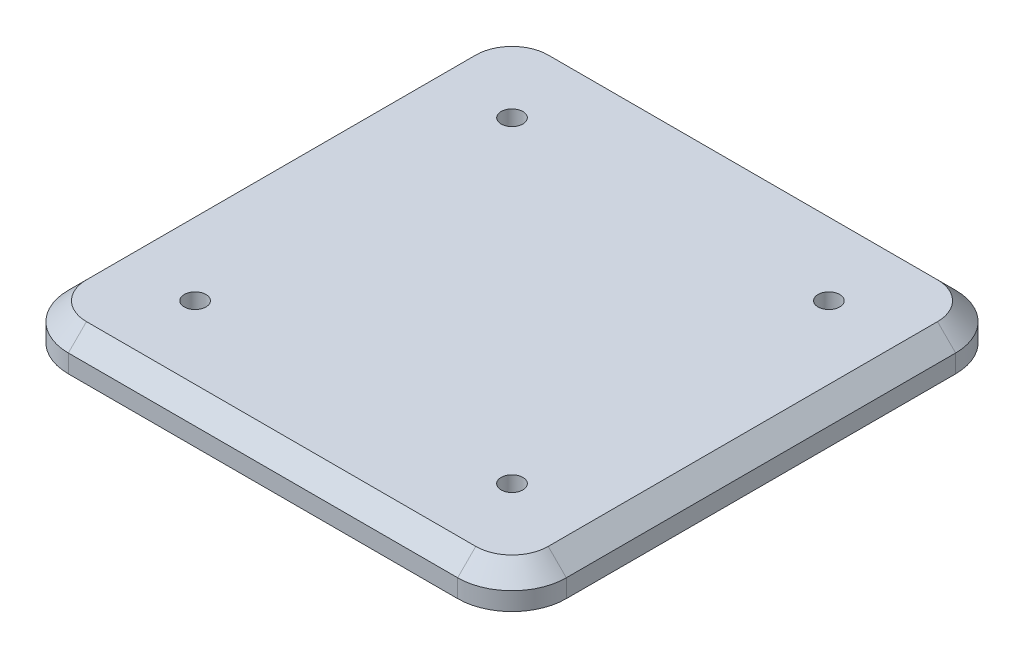
ISO-10303-21;
HEADER;
FILE_DESCRIPTION(('STEP AP214'),'2;1');
FILE_NAME('part.step','',(''),(''),'','','');
FILE_SCHEMA(('AUTOMOTIVE_DESIGN { 1 0 10303 214 1 1 1 1 }'));
ENDSEC;
DATA;
#1=APPLICATION_CONTEXT('core data for automotive mechanical design processes');
#2=APPLICATION_PROTOCOL_DEFINITION('international standard','automotive_design',2000,#1);
#3=PRODUCT_CONTEXT('',#1,'mechanical');
#4=PRODUCT('Part','Part','',(#3));
#5=PRODUCT_RELATED_PRODUCT_CATEGORY('part','',(#4));
#6=PRODUCT_DEFINITION_FORMATION('','',#4);
#7=PRODUCT_DEFINITION_CONTEXT('part definition',#1,'design');
#8=PRODUCT_DEFINITION('design','',#6,#7);
#9=PRODUCT_DEFINITION_SHAPE('','',#8);
#10=(LENGTH_UNIT() NAMED_UNIT(*) SI_UNIT(.MILLI.,.METRE.));
#11=(NAMED_UNIT(*) PLANE_ANGLE_UNIT() SI_UNIT($,.RADIAN.));
#12=(NAMED_UNIT(*) SI_UNIT($,.STERADIAN.) SOLID_ANGLE_UNIT());
#13=UNCERTAINTY_MEASURE_WITH_UNIT(LENGTH_MEASURE(1.E-05),#10,'distance_accuracy_value','');
#14=(GEOMETRIC_REPRESENTATION_CONTEXT(3) GLOBAL_UNCERTAINTY_ASSIGNED_CONTEXT((#13)) GLOBAL_UNIT_ASSIGNED_CONTEXT((#10,
#11,#12)) REPRESENTATION_CONTEXT('',''));
#15=CARTESIAN_POINT('',(0.,0.,0.));
#16=DIRECTION('',(0.,0.,1.));
#17=DIRECTION('',(1.,0.,0.));
#18=AXIS2_PLACEMENT_3D('',#15,#16,#17);
#19=CARTESIAN_POINT('',(-137.5,20.,137.5));
#20=DIRECTION('',(0.,0.,-1.));
#21=DIRECTION('',(-1.,0.,0.));
#22=AXIS2_PLACEMENT_3D('',#19,#20,#21);
#23=PLANE('',#22);
#24=DIRECTION('',(0.,-1.,0.));
#25=VECTOR('',#24,1.);
#26=CARTESIAN_POINT('',(107.5,20.,137.5));
#27=LINE('',#26,#25);
#28=CARTESIAN_POINT('',(107.5,0.,137.5));
#29=VERTEX_POINT('',#28);
#30=CARTESIAN_POINT('',(107.5,9.99999999999999,137.5));
#31=VERTEX_POINT('',#30);
#32=EDGE_CURVE('E249',#29,#31,#27,.F.);
#33=ORIENTED_EDGE('',*,*,#32,.T.);
#34=DIRECTION('',(-1.,0.,0.));
#35=VECTOR('',#34,1.);
#36=CARTESIAN_POINT('',(-107.5,9.99999999999999,137.5));
#37=LINE('',#36,#35);
#38=CARTESIAN_POINT('',(-107.5,9.99999999999999,137.5));
#39=VERTEX_POINT('',#38);
#40=EDGE_CURVE('E11',#31,#39,#37,.T.);
#41=ORIENTED_EDGE('',*,*,#40,.T.);
#42=DIRECTION('',(0.,-1.,0.));
#43=VECTOR('',#42,1.);
#44=CARTESIAN_POINT('',(-107.5,0.,137.5));
#45=LINE('',#44,#43);
#46=CARTESIAN_POINT('',(-107.5,0.,137.5));
#47=VERTEX_POINT('',#46);
#48=EDGE_CURVE('E250',#39,#47,#45,.T.);
#49=ORIENTED_EDGE('',*,*,#48,.T.);
#50=DIRECTION('',(1.,0.,0.));
#51=VECTOR('',#50,1.);
#52=CARTESIAN_POINT('',(-137.5,0.,137.5));
#53=LINE('',#52,#51);
#54=EDGE_CURVE('E215',#47,#29,#53,.T.);
#55=ORIENTED_EDGE('',*,*,#54,.T.);
#56=EDGE_LOOP('',(#33,#41,#49,#55));
#57=FACE_BOUND('',#56,.T.);
#58=ADVANCED_FACE('F41',(#57),#23,.F.);
#59=CARTESIAN_POINT('',(137.5,20.,137.5));
#60=DIRECTION('',(-1.,0.,0.));
#61=DIRECTION('',(0.,0.,1.));
#62=AXIS2_PLACEMENT_3D('',#59,#60,#61);
#63=PLANE('',#62);
#64=DIRECTION('',(0.,-1.,0.));
#65=VECTOR('',#64,1.);
#66=CARTESIAN_POINT('',(137.5,20.,-107.5));
#67=LINE('',#66,#65);
#68=CARTESIAN_POINT('',(137.5,0.,-107.5));
#69=VERTEX_POINT('',#68);
#70=CARTESIAN_POINT('',(137.5,9.99999999999999,-107.5));
#71=VERTEX_POINT('',#70);
#72=EDGE_CURVE('E239',#69,#71,#67,.F.);
#73=ORIENTED_EDGE('',*,*,#72,.T.);
#74=DIRECTION('',(0.,0.,1.));
#75=VECTOR('',#74,1.);
#76=CARTESIAN_POINT('',(137.5,9.99999999999999,107.5));
#77=LINE('',#76,#75);
#78=CARTESIAN_POINT('',(137.5,9.99999999999999,107.5));
#79=VERTEX_POINT('',#78);
#80=EDGE_CURVE('E280',#71,#79,#77,.T.);
#81=ORIENTED_EDGE('',*,*,#80,.T.);
#82=DIRECTION('',(0.,-1.,0.));
#83=VECTOR('',#82,1.);
#84=CARTESIAN_POINT('',(137.5,20.,107.5));
#85=LINE('',#84,#83);
#86=CARTESIAN_POINT('',(137.5,0.,107.5));
#87=VERTEX_POINT('',#86);
#88=EDGE_CURVE('E240',#79,#87,#85,.T.);
#89=ORIENTED_EDGE('',*,*,#88,.T.);
#90=DIRECTION('',(0.,0.,-1.));
#91=VECTOR('',#90,1.);
#92=CARTESIAN_POINT('',(137.5,0.,137.5));
#93=LINE('',#92,#91);
#94=EDGE_CURVE('E214',#87,#69,#93,.T.);
#95=ORIENTED_EDGE('',*,*,#94,.T.);
#96=EDGE_LOOP('',(#73,#81,#89,#95));
#97=FACE_BOUND('',#96,.T.);
#98=ADVANCED_FACE('F349',(#97),#63,.F.);
#99=CARTESIAN_POINT('',(-137.5,20.,-137.5));
#100=DIRECTION('',(0.,0.,-1.));
#101=DIRECTION('',(-1.,0.,0.));
#102=AXIS2_PLACEMENT_3D('',#99,#100,#101);
#103=PLANE('',#102);
#104=DIRECTION('',(0.,-1.,0.));
#105=VECTOR('',#104,1.);
#106=CARTESIAN_POINT('',(-107.5,20.,-137.5));
#107=LINE('',#106,#105);
#108=CARTESIAN_POINT('',(-107.5,0.,-137.5));
#109=VERTEX_POINT('',#108);
#110=CARTESIAN_POINT('',(-107.5,9.99999999999999,-137.5));
#111=VERTEX_POINT('',#110);
#112=EDGE_CURVE('E221',#109,#111,#107,.F.);
#113=ORIENTED_EDGE('',*,*,#112,.T.);
#114=DIRECTION('',(1.,0.,0.));
#115=VECTOR('',#114,1.);
#116=CARTESIAN_POINT('',(-137.5,9.99999999999999,-137.5));
#117=LINE('',#116,#115);
#118=CARTESIAN_POINT('',(107.5,9.99999999999999,-137.5));
#119=VERTEX_POINT('',#118);
#120=EDGE_CURVE('E253',#111,#119,#117,.T.);
#121=ORIENTED_EDGE('',*,*,#120,.T.);
#122=DIRECTION('',(0.,-1.,0.));
#123=VECTOR('',#122,1.);
#124=CARTESIAN_POINT('',(107.5,0.,-137.5));
#125=LINE('',#124,#123);
#126=CARTESIAN_POINT('',(107.5,0.,-137.5));
#127=VERTEX_POINT('',#126);
#128=EDGE_CURVE('E230',#119,#127,#125,.T.);
#129=ORIENTED_EDGE('',*,*,#128,.T.);
#130=DIRECTION('',(1.,0.,0.));
#131=VECTOR('',#130,1.);
#132=CARTESIAN_POINT('',(-137.5,0.,-137.5));
#133=LINE('',#132,#131);
#134=EDGE_CURVE('E217',#109,#127,#133,.T.);
#135=ORIENTED_EDGE('',*,*,#134,.F.);
#136=EDGE_LOOP('',(#113,#121,#129,#135));
#137=FACE_BOUND('',#136,.T.);
#138=ADVANCED_FACE('F332',(#137),#103,.T.);
#139=CARTESIAN_POINT('',(-137.5,20.,137.5));
#140=DIRECTION('',(-1.,0.,0.));
#141=DIRECTION('',(0.,0.,1.));
#142=AXIS2_PLACEMENT_3D('',#139,#140,#141);
#143=PLANE('',#142);
#144=DIRECTION('',(0.,-1.,0.));
#145=VECTOR('',#144,1.);
#146=CARTESIAN_POINT('',(-137.5,20.,107.5));
#147=LINE('',#146,#145);
#148=CARTESIAN_POINT('',(-137.5,0.,107.5));
#149=VERTEX_POINT('',#148);
#150=CARTESIAN_POINT('',(-137.5,9.99999999999999,107.5));
#151=VERTEX_POINT('',#150);
#152=EDGE_CURVE('E245',#149,#151,#147,.F.);
#153=ORIENTED_EDGE('',*,*,#152,.T.);
#154=DIRECTION('',(0.,0.,-1.));
#155=VECTOR('',#154,1.);
#156=CARTESIAN_POINT('',(-137.5,9.99999999999999,137.5));
#157=LINE('',#156,#155);
#158=CARTESIAN_POINT('',(-137.5,9.99999999999999,-107.5));
#159=VERTEX_POINT('',#158);
#160=EDGE_CURVE('E274',#151,#159,#157,.T.);
#161=ORIENTED_EDGE('',*,*,#160,.T.);
#162=DIRECTION('',(0.,-1.,0.));
#163=VECTOR('',#162,1.);
#164=CARTESIAN_POINT('',(-137.5,20.,-107.5));
#165=LINE('',#164,#163);
#166=CARTESIAN_POINT('',(-137.5,0.,-107.5));
#167=VERTEX_POINT('',#166);
#168=EDGE_CURVE('E244',#159,#167,#165,.T.);
#169=ORIENTED_EDGE('',*,*,#168,.T.);
#170=DIRECTION('',(0.,0.,-1.));
#171=VECTOR('',#170,1.);
#172=CARTESIAN_POINT('',(-137.5,0.,137.5));
#173=LINE('',#172,#171);
#174=EDGE_CURVE('E222',#149,#167,#173,.T.);
#175=ORIENTED_EDGE('',*,*,#174,.F.);
#176=EDGE_LOOP('',(#153,#161,#169,#175));
#177=FACE_BOUND('',#176,.T.);
#178=ADVANCED_FACE('F345',(#177),#143,.T.);
#179=CARTESIAN_POINT('',(0.,20.,0.));
#180=DIRECTION('',(0.,1.,0.));
#181=DIRECTION('',(0.,0.,1.));
#182=AXIS2_PLACEMENT_3D('',#179,#180,#181);
#183=PLANE('',#182);
#184=CARTESIAN_POINT('',(-87.5,20.,-87.5));
#185=DIRECTION('',(0.,1.,0.));
#186=DIRECTION('',(0.,0.,1.));
#187=AXIS2_PLACEMENT_3D('',#184,#185,#186);
#188=CIRCLE('',#187,5.99999999999999);
#189=CARTESIAN_POINT('',(-87.5,20.,-81.5));
#190=VERTEX_POINT('',#189);
#191=EDGE_CURVE('E190',#190,#190,#188,.T.);
#192=ORIENTED_EDGE('',*,*,#191,.F.);
#193=EDGE_LOOP('',(#192));
#194=FACE_BOUND('',#193,.T.);
#195=CARTESIAN_POINT('',(87.5,20.,-87.5));
#196=DIRECTION('',(0.,1.,0.));
#197=DIRECTION('',(0.,0.,1.));
#198=AXIS2_PLACEMENT_3D('',#195,#196,#197);
#199=CIRCLE('',#198,5.99999999999999);
#200=CARTESIAN_POINT('',(87.5,20.,-81.5));
#201=VERTEX_POINT('',#200);
#202=EDGE_CURVE('E191',#201,#201,#199,.T.);
#203=ORIENTED_EDGE('',*,*,#202,.F.);
#204=EDGE_LOOP('',(#203));
#205=FACE_BOUND('',#204,.T.);
#206=CARTESIAN_POINT('',(87.5,20.,87.5));
#207=DIRECTION('',(0.,1.,0.));
#208=DIRECTION('',(0.,0.,1.));
#209=AXIS2_PLACEMENT_3D('',#206,#207,#208);
#210=CIRCLE('',#209,5.99999999999999);
#211=CARTESIAN_POINT('',(87.5,20.,93.5));
#212=VERTEX_POINT('',#211);
#213=EDGE_CURVE('E200',#212,#212,#210,.T.);
#214=ORIENTED_EDGE('',*,*,#213,.F.);
#215=EDGE_LOOP('',(#214));
#216=FACE_BOUND('',#215,.T.);
#217=CARTESIAN_POINT('',(-87.5,20.,87.5));
#218=DIRECTION('',(0.,1.,0.));
#219=DIRECTION('',(0.,0.,1.));
#220=AXIS2_PLACEMENT_3D('',#217,#218,#219);
#221=CIRCLE('',#220,5.99999999999999);
#222=CARTESIAN_POINT('',(-87.5,20.,93.5));
#223=VERTEX_POINT('',#222);
#224=EDGE_CURVE('E202',#223,#223,#221,.T.);
#225=ORIENTED_EDGE('',*,*,#224,.F.);
#226=EDGE_LOOP('',(#225));
#227=FACE_BOUND('',#226,.T.);
#228=CARTESIAN_POINT('',(107.5,20.,-107.5));
#229=DIRECTION('',(0.,1.,0.));
#230=DIRECTION('',(0.,0.,1.));
#231=AXIS2_PLACEMENT_3D('',#228,#229,#230);
#232=CIRCLE('',#231,20.);
#233=CARTESIAN_POINT('',(127.5,20.,-107.5));
#234=VERTEX_POINT('',#233);
#235=CARTESIAN_POINT('',(107.5,20.,-127.5));
#236=VERTEX_POINT('',#235);
#237=EDGE_CURVE('E262',#234,#236,#232,.T.);
#238=ORIENTED_EDGE('',*,*,#237,.T.);
#239=DIRECTION('',(-1.,0.,0.));
#240=VECTOR('',#239,1.);
#241=CARTESIAN_POINT('',(0.,20.,-127.5));
#242=LINE('',#241,#240);
#243=CARTESIAN_POINT('',(-107.5,20.,-127.5));
#244=VERTEX_POINT('',#243);
#245=EDGE_CURVE('E268',#236,#244,#242,.T.);
#246=ORIENTED_EDGE('',*,*,#245,.T.);
#247=CARTESIAN_POINT('',(-107.5,20.,-107.5));
#248=DIRECTION('',(0.,1.,0.));
#249=DIRECTION('',(0.,0.,1.));
#250=AXIS2_PLACEMENT_3D('',#247,#248,#249);
#251=CIRCLE('',#250,20.);
#252=CARTESIAN_POINT('',(-127.5,20.,-107.5));
#253=VERTEX_POINT('',#252);
#254=EDGE_CURVE('E266',#244,#253,#251,.T.);
#255=ORIENTED_EDGE('',*,*,#254,.T.);
#256=DIRECTION('',(0.,0.,1.));
#257=VECTOR('',#256,1.);
#258=CARTESIAN_POINT('',(-127.5,20.,0.));
#259=LINE('',#258,#257);
#260=CARTESIAN_POINT('',(-127.5,20.,107.5));
#261=VERTEX_POINT('',#260);
#262=EDGE_CURVE('E265',#253,#261,#259,.T.);
#263=ORIENTED_EDGE('',*,*,#262,.T.);
#264=CARTESIAN_POINT('',(-107.5,20.,107.5));
#265=DIRECTION('',(0.,1.,0.));
#266=DIRECTION('',(0.,0.,1.));
#267=AXIS2_PLACEMENT_3D('',#264,#265,#266);
#268=CIRCLE('',#267,20.);
#269=CARTESIAN_POINT('',(-107.5,20.,127.5));
#270=VERTEX_POINT('',#269);
#271=EDGE_CURVE('E256',#261,#270,#268,.T.);
#272=ORIENTED_EDGE('',*,*,#271,.T.);
#273=DIRECTION('',(1.,0.,0.));
#274=VECTOR('',#273,1.);
#275=CARTESIAN_POINT('',(107.5,20.,127.5));
#276=LINE('',#275,#274);
#277=CARTESIAN_POINT('',(107.5,20.,127.5));
#278=VERTEX_POINT('',#277);
#279=EDGE_CURVE('E255',#270,#278,#276,.T.);
#280=ORIENTED_EDGE('',*,*,#279,.T.);
#281=CARTESIAN_POINT('',(107.5,20.,107.5));
#282=DIRECTION('',(0.,1.,0.));
#283=DIRECTION('',(0.,0.,1.));
#284=AXIS2_PLACEMENT_3D('',#281,#282,#283);
#285=CIRCLE('',#284,20.);
#286=CARTESIAN_POINT('',(127.5,20.,107.5));
#287=VERTEX_POINT('',#286);
#288=EDGE_CURVE('E258',#278,#287,#285,.T.);
#289=ORIENTED_EDGE('',*,*,#288,.T.);
#290=DIRECTION('',(0.,0.,-1.));
#291=VECTOR('',#290,1.);
#292=CARTESIAN_POINT('',(127.5,20.,-107.5));
#293=LINE('',#292,#291);
#294=EDGE_CURVE('E257',#287,#234,#293,.T.);
#295=ORIENTED_EDGE('',*,*,#294,.T.);
#296=EDGE_LOOP('',(#238,#246,#255,#263,#272,#280,#289,#295));
#297=FACE_BOUND('',#296,.T.);
#298=ADVANCED_FACE('F313',(#194,#205,#216,#227,#297),#183,.T.);
#299=CARTESIAN_POINT('',(0.,0.,0.));
#300=DIRECTION('',(0.,1.,0.));
#301=DIRECTION('',(0.,0.,1.));
#302=AXIS2_PLACEMENT_3D('',#299,#300,#301);
#303=PLANE('',#302);
#304=CARTESIAN_POINT('',(-112.5,0.,112.5));
#305=DIRECTION('',(0.,-1.,0.));
#306=DIRECTION('',(0.,0.,-1.));
#307=AXIS2_PLACEMENT_3D('',#304,#305,#306);
#308=CIRCLE('',#307,5.99999999999999);
#309=CARTESIAN_POINT('',(-112.5,0.,106.5));
#310=VERTEX_POINT('',#309);
#311=EDGE_CURVE('E164',#310,#310,#308,.T.);
#312=ORIENTED_EDGE('',*,*,#311,.F.);
#313=EDGE_LOOP('',(#312));
#314=FACE_BOUND('',#313,.T.);
#315=CARTESIAN_POINT('',(112.5,0.,112.5));
#316=DIRECTION('',(0.,-1.,0.));
#317=DIRECTION('',(0.,0.,-1.));
#318=AXIS2_PLACEMENT_3D('',#315,#316,#317);
#319=CIRCLE('',#318,5.99999999999999);
#320=CARTESIAN_POINT('',(112.5,0.,106.5));
#321=VERTEX_POINT('',#320);
#322=EDGE_CURVE('E163',#321,#321,#319,.T.);
#323=ORIENTED_EDGE('',*,*,#322,.F.);
#324=EDGE_LOOP('',(#323));
#325=FACE_BOUND('',#324,.T.);
#326=CARTESIAN_POINT('',(112.5,0.,-112.5));
#327=DIRECTION('',(0.,-1.,0.));
#328=DIRECTION('',(0.,0.,-1.));
#329=AXIS2_PLACEMENT_3D('',#326,#327,#328);
#330=CIRCLE('',#329,5.99999999999999);
#331=CARTESIAN_POINT('',(112.5,0.,-118.5));
#332=VERTEX_POINT('',#331);
#333=EDGE_CURVE('E174',#332,#332,#330,.T.);
#334=ORIENTED_EDGE('',*,*,#333,.F.);
#335=EDGE_LOOP('',(#334));
#336=FACE_BOUND('',#335,.T.);
#337=CARTESIAN_POINT('',(-112.5,0.,-112.5));
#338=DIRECTION('',(0.,-1.,0.));
#339=DIRECTION('',(0.,0.,-1.));
#340=AXIS2_PLACEMENT_3D('',#337,#338,#339);
#341=CIRCLE('',#340,5.99999999999999);
#342=CARTESIAN_POINT('',(-112.5,0.,-118.5));
#343=VERTEX_POINT('',#342);
#344=EDGE_CURVE('E182',#343,#343,#341,.T.);
#345=ORIENTED_EDGE('',*,*,#344,.F.);
#346=EDGE_LOOP('',(#345));
#347=FACE_BOUND('',#346,.T.);
#348=ORIENTED_EDGE('',*,*,#134,.T.);
#349=CARTESIAN_POINT('',(107.5,0.,-107.5));
#350=DIRECTION('',(0.,1.,0.));
#351=DIRECTION('',(0.,0.,1.));
#352=AXIS2_PLACEMENT_3D('',#349,#350,#351);
#353=CIRCLE('',#352,30.);
#354=EDGE_CURVE('E232',#127,#69,#353,.F.);
#355=ORIENTED_EDGE('',*,*,#354,.T.);
#356=ORIENTED_EDGE('',*,*,#94,.F.);
#357=CARTESIAN_POINT('',(107.5,0.,107.5));
#358=DIRECTION('',(0.,1.,0.));
#359=DIRECTION('',(0.,0.,1.));
#360=AXIS2_PLACEMENT_3D('',#357,#358,#359);
#361=CIRCLE('',#360,30.);
#362=EDGE_CURVE('E233',#87,#29,#361,.F.);
#363=ORIENTED_EDGE('',*,*,#362,.T.);
#364=ORIENTED_EDGE('',*,*,#54,.F.);
#365=CARTESIAN_POINT('',(-107.5,0.,107.5));
#366=DIRECTION('',(0.,1.,0.));
#367=DIRECTION('',(0.,0.,1.));
#368=AXIS2_PLACEMENT_3D('',#365,#366,#367);
#369=CIRCLE('',#368,30.);
#370=EDGE_CURVE('E227',#47,#149,#369,.F.);
#371=ORIENTED_EDGE('',*,*,#370,.T.);
#372=ORIENTED_EDGE('',*,*,#174,.T.);
#373=CARTESIAN_POINT('',(-107.5,0.,-107.5));
#374=DIRECTION('',(0.,1.,0.));
#375=DIRECTION('',(0.,0.,1.));
#376=AXIS2_PLACEMENT_3D('',#373,#374,#375);
#377=CIRCLE('',#376,30.);
#378=EDGE_CURVE('E231',#167,#109,#377,.F.);
#379=ORIENTED_EDGE('',*,*,#378,.T.);
#380=EDGE_LOOP('',(#348,#355,#356,#363,#364,#371,#372,#379));
#381=FACE_BOUND('',#380,.T.);
#382=ADVANCED_FACE('F333',(#314,#325,#336,#347,#381),#303,.F.);
#383=CARTESIAN_POINT('',(107.5,20.,-107.5));
#384=DIRECTION('',(0.,1.,0.));
#385=DIRECTION('',(0.,0.,1.));
#386=AXIS2_PLACEMENT_3D('',#383,#384,#385);
#387=CYLINDRICAL_SURFACE('',#386,30.);
#388=ORIENTED_EDGE('',*,*,#128,.F.);
#389=CARTESIAN_POINT('',(107.5,9.99999999999999,-107.5));
#390=DIRECTION('',(0.,1.,0.));
#391=DIRECTION('',(0.,0.,1.));
#392=AXIS2_PLACEMENT_3D('',#389,#390,#391);
#393=CIRCLE('',#392,30.);
#394=EDGE_CURVE('E272',#119,#71,#393,.F.);
#395=ORIENTED_EDGE('',*,*,#394,.T.);
#396=ORIENTED_EDGE('',*,*,#72,.F.);
#397=ORIENTED_EDGE('',*,*,#354,.F.);
#398=EDGE_LOOP('',(#388,#395,#396,#397));
#399=FACE_BOUND('',#398,.T.);
#400=ADVANCED_FACE('F355',(#399),#387,.T.);
#401=CARTESIAN_POINT('',(-107.5,20.,-107.5));
#402=DIRECTION('',(0.,-1.,0.));
#403=DIRECTION('',(0.,0.,-1.));
#404=AXIS2_PLACEMENT_3D('',#401,#402,#403);
#405=CYLINDRICAL_SURFACE('',#404,30.);
#406=ORIENTED_EDGE('',*,*,#168,.F.);
#407=CARTESIAN_POINT('',(-107.5,9.99999999999999,-107.5));
#408=DIRECTION('',(0.,1.,0.));
#409=DIRECTION('',(0.,0.,1.));
#410=AXIS2_PLACEMENT_3D('',#407,#408,#409);
#411=CIRCLE('',#410,30.);
#412=EDGE_CURVE('E271',#159,#111,#411,.F.);
#413=ORIENTED_EDGE('',*,*,#412,.T.);
#414=ORIENTED_EDGE('',*,*,#112,.F.);
#415=ORIENTED_EDGE('',*,*,#378,.F.);
#416=EDGE_LOOP('',(#406,#413,#414,#415));
#417=FACE_BOUND('',#416,.T.);
#418=ADVANCED_FACE('F330',(#417),#405,.T.);
#419=CARTESIAN_POINT('',(107.5,20.,107.5));
#420=DIRECTION('',(0.,-1.,0.));
#421=DIRECTION('',(0.,0.,-1.));
#422=AXIS2_PLACEMENT_3D('',#419,#420,#421);
#423=CYLINDRICAL_SURFACE('',#422,30.);
#424=ORIENTED_EDGE('',*,*,#88,.F.);
#425=CARTESIAN_POINT('',(107.5,9.99999999999999,107.5));
#426=DIRECTION('',(0.,1.,0.));
#427=DIRECTION('',(0.,0.,1.));
#428=AXIS2_PLACEMENT_3D('',#425,#426,#427);
#429=CIRCLE('',#428,30.);
#430=EDGE_CURVE('E51',#79,#31,#429,.F.);
#431=ORIENTED_EDGE('',*,*,#430,.T.);
#432=ORIENTED_EDGE('',*,*,#32,.F.);
#433=ORIENTED_EDGE('',*,*,#362,.F.);
#434=EDGE_LOOP('',(#424,#431,#432,#433));
#435=FACE_BOUND('',#434,.T.);
#436=ADVANCED_FACE('F347',(#435),#423,.T.);
#437=CARTESIAN_POINT('',(-107.5,20.,107.5));
#438=DIRECTION('',(0.,1.,0.));
#439=DIRECTION('',(0.,0.,1.));
#440=AXIS2_PLACEMENT_3D('',#437,#438,#439);
#441=CYLINDRICAL_SURFACE('',#440,30.);
#442=ORIENTED_EDGE('',*,*,#48,.F.);
#443=CARTESIAN_POINT('',(-107.5,9.99999999999999,107.5));
#444=DIRECTION('',(0.,1.,0.));
#445=DIRECTION('',(0.,0.,1.));
#446=AXIS2_PLACEMENT_3D('',#443,#444,#445);
#447=CIRCLE('',#446,30.);
#448=EDGE_CURVE('E276',#39,#151,#447,.F.);
#449=ORIENTED_EDGE('',*,*,#448,.T.);
#450=ORIENTED_EDGE('',*,*,#152,.F.);
#451=ORIENTED_EDGE('',*,*,#370,.F.);
#452=EDGE_LOOP('',(#442,#449,#450,#451));
#453=FACE_BOUND('',#452,.T.);
#454=ADVANCED_FACE('F344',(#453),#441,.T.);
#455=CARTESIAN_POINT('',(0.,20.,127.5));
#456=DIRECTION('',(0.,0.707106781186547,0.707106781186547));
#457=DIRECTION('',(-1.,0.,0.));
#458=AXIS2_PLACEMENT_3D('',#455,#456,#457);
#459=PLANE('',#458);
#460=DIRECTION('',(0.,-0.707106781186547,0.707106781186547));
#461=VECTOR('',#460,1.);
#462=CARTESIAN_POINT('',(107.5,20.,127.5));
#463=LINE('',#462,#461);
#464=EDGE_CURVE('E298',#278,#31,#463,.T.);
#465=ORIENTED_EDGE('',*,*,#464,.F.);
#466=ORIENTED_EDGE('',*,*,#279,.F.);
#467=DIRECTION('',(0.,0.707106781186547,-0.707106781186547));
#468=VECTOR('',#467,1.);
#469=CARTESIAN_POINT('',(-107.5,9.99999999999999,137.5));
#470=LINE('',#469,#468);
#471=EDGE_CURVE('E46',#39,#270,#470,.T.);
#472=ORIENTED_EDGE('',*,*,#471,.F.);
#473=ORIENTED_EDGE('',*,*,#40,.F.);
#474=EDGE_LOOP('',(#465,#466,#472,#473));
#475=FACE_BOUND('',#474,.T.);
#476=ADVANCED_FACE('F42',(#475),#459,.T.);
#477=CARTESIAN_POINT('',(-107.5,20.,107.5));
#478=DIRECTION('',(0.,-1.,0.));
#479=DIRECTION('',(0.,0.,-1.));
#480=AXIS2_PLACEMENT_3D('',#477,#478,#479);
#481=CONICAL_SURFACE('',#480,20.,0.785398163397448);
#482=ORIENTED_EDGE('',*,*,#471,.T.);
#483=ORIENTED_EDGE('',*,*,#271,.F.);
#484=DIRECTION('',(0.707106781186547,0.707106781186547,0.));
#485=VECTOR('',#484,1.);
#486=CARTESIAN_POINT('',(-137.5,9.99999999999999,107.5));
#487=LINE('',#486,#485);
#488=EDGE_CURVE('E294',#151,#261,#487,.T.);
#489=ORIENTED_EDGE('',*,*,#488,.F.);
#490=ORIENTED_EDGE('',*,*,#448,.F.);
#491=EDGE_LOOP('',(#482,#483,#489,#490));
#492=FACE_BOUND('',#491,.T.);
#493=ADVANCED_FACE('F308',(#492),#481,.T.);
#494=CARTESIAN_POINT('',(107.5,20.,107.5));
#495=DIRECTION('',(0.,-1.,0.));
#496=DIRECTION('',(0.,0.,-1.));
#497=AXIS2_PLACEMENT_3D('',#494,#495,#496);
#498=CONICAL_SURFACE('',#497,20.,0.785398163397448);
#499=ORIENTED_EDGE('',*,*,#464,.T.);
#500=ORIENTED_EDGE('',*,*,#430,.F.);
#501=DIRECTION('',(0.707106781186547,-0.707106781186547,0.));
#502=VECTOR('',#501,1.);
#503=CARTESIAN_POINT('',(127.5,20.,107.5));
#504=LINE('',#503,#502);
#505=EDGE_CURVE('E292',#287,#79,#504,.T.);
#506=ORIENTED_EDGE('',*,*,#505,.F.);
#507=ORIENTED_EDGE('',*,*,#288,.F.);
#508=EDGE_LOOP('',(#499,#500,#506,#507));
#509=FACE_BOUND('',#508,.T.);
#510=ADVANCED_FACE('F362',(#509),#498,.T.);
#511=CARTESIAN_POINT('',(-137.5,9.99999999999999,137.5));
#512=DIRECTION('',(0.707106781186547,-0.707106781186547,0.));
#513=DIRECTION('',(0.,0.,-1.));
#514=AXIS2_PLACEMENT_3D('',#511,#512,#513);
#515=PLANE('',#514);
#516=ORIENTED_EDGE('',*,*,#488,.T.);
#517=ORIENTED_EDGE('',*,*,#262,.F.);
#518=DIRECTION('',(0.707106781186547,0.707106781186547,0.));
#519=VECTOR('',#518,1.);
#520=CARTESIAN_POINT('',(-137.5,9.99999999999999,-107.5));
#521=LINE('',#520,#519);
#522=EDGE_CURVE('E286',#159,#253,#521,.T.);
#523=ORIENTED_EDGE('',*,*,#522,.F.);
#524=ORIENTED_EDGE('',*,*,#160,.F.);
#525=EDGE_LOOP('',(#516,#517,#523,#524));
#526=FACE_BOUND('',#525,.T.);
#527=ADVANCED_FACE('F320',(#526),#515,.F.);
#528=CARTESIAN_POINT('',(127.5,20.,0.));
#529=DIRECTION('',(0.707106781186547,0.707106781186547,0.));
#530=DIRECTION('',(0.,0.,1.));
#531=AXIS2_PLACEMENT_3D('',#528,#529,#530);
#532=PLANE('',#531);
#533=ORIENTED_EDGE('',*,*,#505,.T.);
#534=ORIENTED_EDGE('',*,*,#80,.F.);
#535=DIRECTION('',(0.707106781186547,-0.707106781186547,0.));
#536=VECTOR('',#535,1.);
#537=CARTESIAN_POINT('',(127.5,20.,-107.5));
#538=LINE('',#537,#536);
#539=EDGE_CURVE('E284',#234,#71,#538,.T.);
#540=ORIENTED_EDGE('',*,*,#539,.F.);
#541=ORIENTED_EDGE('',*,*,#294,.F.);
#542=EDGE_LOOP('',(#533,#534,#540,#541));
#543=FACE_BOUND('',#542,.T.);
#544=ADVANCED_FACE('F363',(#543),#532,.T.);
#545=CARTESIAN_POINT('',(-107.5,20.,-107.5));
#546=DIRECTION('',(0.,-1.,0.));
#547=DIRECTION('',(0.,0.,-1.));
#548=AXIS2_PLACEMENT_3D('',#545,#546,#547);
#549=CONICAL_SURFACE('',#548,20.,0.785398163397448);
#550=ORIENTED_EDGE('',*,*,#522,.T.);
#551=ORIENTED_EDGE('',*,*,#254,.F.);
#552=DIRECTION('',(0.,0.707106781186547,0.707106781186547));
#553=VECTOR('',#552,1.);
#554=CARTESIAN_POINT('',(-107.5,9.99999999999999,-137.5));
#555=LINE('',#554,#553);
#556=EDGE_CURVE('E281',#111,#244,#555,.T.);
#557=ORIENTED_EDGE('',*,*,#556,.F.);
#558=ORIENTED_EDGE('',*,*,#412,.F.);
#559=EDGE_LOOP('',(#550,#551,#557,#558));
#560=FACE_BOUND('',#559,.T.);
#561=ADVANCED_FACE('F321',(#560),#549,.T.);
#562=CARTESIAN_POINT('',(107.5,20.,-107.5));
#563=DIRECTION('',(0.,-1.,0.));
#564=DIRECTION('',(0.,0.,-1.));
#565=AXIS2_PLACEMENT_3D('',#562,#563,#564);
#566=CONICAL_SURFACE('',#565,20.,0.785398163397448);
#567=ORIENTED_EDGE('',*,*,#539,.T.);
#568=ORIENTED_EDGE('',*,*,#394,.F.);
#569=DIRECTION('',(0.,-0.707106781186547,-0.707106781186547));
#570=VECTOR('',#569,1.);
#571=CARTESIAN_POINT('',(107.5,20.,-127.5));
#572=LINE('',#571,#570);
#573=EDGE_CURVE('E211',#236,#119,#572,.T.);
#574=ORIENTED_EDGE('',*,*,#573,.F.);
#575=ORIENTED_EDGE('',*,*,#237,.F.);
#576=EDGE_LOOP('',(#567,#568,#574,#575));
#577=FACE_BOUND('',#576,.T.);
#578=ADVANCED_FACE('F358',(#577),#566,.T.);
#579=CARTESIAN_POINT('',(-137.5,9.99999999999999,-137.5));
#580=DIRECTION('',(0.,-0.707106781186547,0.707106781186547));
#581=DIRECTION('',(1.,0.,0.));
#582=AXIS2_PLACEMENT_3D('',#579,#580,#581);
#583=PLANE('',#582);
#584=ORIENTED_EDGE('',*,*,#556,.T.);
#585=ORIENTED_EDGE('',*,*,#245,.F.);
#586=ORIENTED_EDGE('',*,*,#573,.T.);
#587=ORIENTED_EDGE('',*,*,#120,.F.);
#588=EDGE_LOOP('',(#584,#585,#586,#587));
#589=FACE_BOUND('',#588,.T.);
#590=ADVANCED_FACE('F389',(#589),#583,.F.);
#591=CARTESIAN_POINT('',(-87.5,10.,87.5));
#592=DIRECTION('',(0.,1.,0.));
#593=DIRECTION('',(0.,0.,1.));
#594=AXIS2_PLACEMENT_3D('',#591,#592,#593);
#595=CONICAL_SURFACE('',#594,5.99999999999999,1.02974425867665);
#596=CARTESIAN_POINT('',(-87.5,6.39483628583465,87.5));
#597=VERTEX_POINT('',#596);
#598=VERTEX_LOOP('',#597);
#599=FACE_BOUND('',#598,.T.);
#600=CARTESIAN_POINT('',(-87.5,10.,87.5));
#601=DIRECTION('',(0.,1.,0.));
#602=DIRECTION('',(0.,0.,1.));
#603=AXIS2_PLACEMENT_3D('',#600,#601,#602);
#604=CIRCLE('',#603,5.99999999999999);
#605=CARTESIAN_POINT('',(-87.5,10.,93.5));
#606=VERTEX_POINT('',#605);
#607=EDGE_CURVE('E208',#606,#606,#604,.T.);
#608=ORIENTED_EDGE('',*,*,#607,.T.);
#609=EDGE_LOOP('',(#608));
#610=FACE_BOUND('',#609,.T.);
#611=ADVANCED_FACE('F392',(#599,#610),#595,.F.);
#612=CARTESIAN_POINT('',(-87.5,20.,87.5));
#613=DIRECTION('',(0.,1.,0.));
#614=DIRECTION('',(0.,0.,1.));
#615=AXIS2_PLACEMENT_3D('',#612,#613,#614);
#616=CYLINDRICAL_SURFACE('',#615,5.99999999999999);
#617=ORIENTED_EDGE('',*,*,#607,.F.);
#618=EDGE_LOOP('',(#617));
#619=FACE_BOUND('',#618,.T.);
#620=ORIENTED_EDGE('',*,*,#224,.T.);
#621=EDGE_LOOP('',(#620));
#622=FACE_BOUND('',#621,.T.);
#623=ADVANCED_FACE('F452',(#619,#622),#616,.F.);
#624=CARTESIAN_POINT('',(87.5,10.,87.5));
#625=DIRECTION('',(0.,1.,0.));
#626=DIRECTION('',(0.,0.,1.));
#627=AXIS2_PLACEMENT_3D('',#624,#625,#626);
#628=CONICAL_SURFACE('',#627,5.99999999999999,1.02974425867665);
#629=CARTESIAN_POINT('',(87.5,6.39483628583465,87.5));
#630=VERTEX_POINT('',#629);
#631=VERTEX_LOOP('',#630);
#632=FACE_BOUND('',#631,.T.);
#633=CARTESIAN_POINT('',(87.5,10.,87.5));
#634=DIRECTION('',(0.,1.,0.));
#635=DIRECTION('',(0.,0.,1.));
#636=AXIS2_PLACEMENT_3D('',#633,#634,#635);
#637=CIRCLE('',#636,5.99999999999999);
#638=CARTESIAN_POINT('',(87.5,10.,93.5));
#639=VERTEX_POINT('',#638);
#640=EDGE_CURVE('E205',#639,#639,#637,.T.);
#641=ORIENTED_EDGE('',*,*,#640,.T.);
#642=EDGE_LOOP('',(#641));
#643=FACE_BOUND('',#642,.T.);
#644=ADVANCED_FACE('F462',(#632,#643),#628,.F.);
#645=CARTESIAN_POINT('',(87.5,20.,87.5));
#646=DIRECTION('',(0.,1.,0.));
#647=DIRECTION('',(0.,0.,1.));
#648=AXIS2_PLACEMENT_3D('',#645,#646,#647);
#649=CYLINDRICAL_SURFACE('',#648,5.99999999999999);
#650=ORIENTED_EDGE('',*,*,#640,.F.);
#651=EDGE_LOOP('',(#650));
#652=FACE_BOUND('',#651,.T.);
#653=ORIENTED_EDGE('',*,*,#213,.T.);
#654=EDGE_LOOP('',(#653));
#655=FACE_BOUND('',#654,.T.);
#656=ADVANCED_FACE('F471',(#652,#655),#649,.F.);
#657=CARTESIAN_POINT('',(87.5,10.,-87.5));
#658=DIRECTION('',(0.,1.,0.));
#659=DIRECTION('',(0.,0.,1.));
#660=AXIS2_PLACEMENT_3D('',#657,#658,#659);
#661=CONICAL_SURFACE('',#660,5.99999999999999,1.02974425867665);
#662=CARTESIAN_POINT('',(87.5,6.39483628583465,-87.5));
#663=VERTEX_POINT('',#662);
#664=VERTEX_LOOP('',#663);
#665=FACE_BOUND('',#664,.T.);
#666=CARTESIAN_POINT('',(87.5,10.,-87.5));
#667=DIRECTION('',(0.,1.,0.));
#668=DIRECTION('',(0.,0.,1.));
#669=AXIS2_PLACEMENT_3D('',#666,#667,#668);
#670=CIRCLE('',#669,5.99999999999999);
#671=CARTESIAN_POINT('',(87.5,10.,-81.5));
#672=VERTEX_POINT('',#671);
#673=EDGE_CURVE('E198',#672,#672,#670,.T.);
#674=ORIENTED_EDGE('',*,*,#673,.T.);
#675=EDGE_LOOP('',(#674));
#676=FACE_BOUND('',#675,.T.);
#677=ADVANCED_FACE('F485',(#665,#676),#661,.F.);
#678=CARTESIAN_POINT('',(87.5,20.,-87.5));
#679=DIRECTION('',(0.,1.,0.));
#680=DIRECTION('',(0.,0.,1.));
#681=AXIS2_PLACEMENT_3D('',#678,#679,#680);
#682=CYLINDRICAL_SURFACE('',#681,5.99999999999999);
#683=ORIENTED_EDGE('',*,*,#673,.F.);
#684=EDGE_LOOP('',(#683));
#685=FACE_BOUND('',#684,.T.);
#686=ORIENTED_EDGE('',*,*,#202,.T.);
#687=EDGE_LOOP('',(#686));
#688=FACE_BOUND('',#687,.T.);
#689=ADVANCED_FACE('F491',(#685,#688),#682,.F.);
#690=CARTESIAN_POINT('',(-87.5,10.,-87.5));
#691=DIRECTION('',(0.,1.,0.));
#692=DIRECTION('',(0.,0.,1.));
#693=AXIS2_PLACEMENT_3D('',#690,#691,#692);
#694=CONICAL_SURFACE('',#693,5.99999999999999,1.02974425867665);
#695=CARTESIAN_POINT('',(-87.5,6.39483628583465,-87.5));
#696=VERTEX_POINT('',#695);
#697=VERTEX_LOOP('',#696);
#698=FACE_BOUND('',#697,.T.);
#699=CARTESIAN_POINT('',(-87.5,10.,-87.5));
#700=DIRECTION('',(0.,1.,0.));
#701=DIRECTION('',(0.,0.,1.));
#702=AXIS2_PLACEMENT_3D('',#699,#700,#701);
#703=CIRCLE('',#702,5.99999999999999);
#704=CARTESIAN_POINT('',(-87.5,10.,-81.5));
#705=VERTEX_POINT('',#704);
#706=EDGE_CURVE('E189',#705,#705,#703,.T.);
#707=ORIENTED_EDGE('',*,*,#706,.T.);
#708=EDGE_LOOP('',(#707));
#709=FACE_BOUND('',#708,.T.);
#710=ADVANCED_FACE('F498',(#698,#709),#694,.F.);
#711=CARTESIAN_POINT('',(-87.5,20.,-87.5));
#712=DIRECTION('',(0.,1.,0.));
#713=DIRECTION('',(0.,0.,1.));
#714=AXIS2_PLACEMENT_3D('',#711,#712,#713);
#715=CYLINDRICAL_SURFACE('',#714,5.99999999999999);
#716=ORIENTED_EDGE('',*,*,#706,.F.);
#717=EDGE_LOOP('',(#716));
#718=FACE_BOUND('',#717,.T.);
#719=ORIENTED_EDGE('',*,*,#191,.T.);
#720=EDGE_LOOP('',(#719));
#721=FACE_BOUND('',#720,.T.);
#722=ADVANCED_FACE('F509',(#718,#721),#715,.F.);
#723=CARTESIAN_POINT('',(-112.5,9.99999999999999,-112.5));
#724=DIRECTION('',(0.,-1.,0.));
#725=DIRECTION('',(0.,0.,-1.));
#726=AXIS2_PLACEMENT_3D('',#723,#724,#725);
#727=CONICAL_SURFACE('',#726,5.99999999999999,1.02974425867665);
#728=CARTESIAN_POINT('',(-112.5,13.6051637141654,-112.5));
#729=VERTEX_POINT('',#728);
#730=VERTEX_LOOP('',#729);
#731=FACE_BOUND('',#730,.T.);
#732=CARTESIAN_POINT('',(-112.5,9.99999999999999,-112.5));
#733=DIRECTION('',(0.,-1.,0.));
#734=DIRECTION('',(0.,0.,-1.));
#735=AXIS2_PLACEMENT_3D('',#732,#733,#734);
#736=CIRCLE('',#735,5.99999999999999);
#737=CARTESIAN_POINT('',(-112.5,9.99999999999999,-118.5));
#738=VERTEX_POINT('',#737);
#739=EDGE_CURVE('E184',#738,#738,#736,.T.);
#740=ORIENTED_EDGE('',*,*,#739,.T.);
#741=EDGE_LOOP('',(#740));
#742=FACE_BOUND('',#741,.T.);
#743=ADVANCED_FACE('F516',(#731,#742),#727,.F.);
#744=CARTESIAN_POINT('',(-112.5,0.,-112.5));
#745=DIRECTION('',(0.,-1.,0.));
#746=DIRECTION('',(0.,0.,-1.));
#747=AXIS2_PLACEMENT_3D('',#744,#745,#746);
#748=CYLINDRICAL_SURFACE('',#747,5.99999999999999);
#749=ORIENTED_EDGE('',*,*,#739,.F.);
#750=EDGE_LOOP('',(#749));
#751=FACE_BOUND('',#750,.T.);
#752=ORIENTED_EDGE('',*,*,#344,.T.);
#753=EDGE_LOOP('',(#752));
#754=FACE_BOUND('',#753,.T.);
#755=ADVANCED_FACE('F532',(#751,#754),#748,.F.);
#756=CARTESIAN_POINT('',(112.5,9.99999999999999,-112.5));
#757=DIRECTION('',(0.,-1.,0.));
#758=DIRECTION('',(0.,0.,-1.));
#759=AXIS2_PLACEMENT_3D('',#756,#757,#758);
#760=CONICAL_SURFACE('',#759,5.99999999999999,1.02974425867665);
#761=CARTESIAN_POINT('',(112.5,13.6051637141654,-112.5));
#762=VERTEX_POINT('',#761);
#763=VERTEX_LOOP('',#762);
#764=FACE_BOUND('',#763,.T.);
#765=CARTESIAN_POINT('',(112.5,9.99999999999999,-112.5));
#766=DIRECTION('',(0.,-1.,0.));
#767=DIRECTION('',(0.,0.,-1.));
#768=AXIS2_PLACEMENT_3D('',#765,#766,#767);
#769=CIRCLE('',#768,5.99999999999999);
#770=CARTESIAN_POINT('',(112.5,9.99999999999999,-118.5));
#771=VERTEX_POINT('',#770);
#772=EDGE_CURVE('E176',#771,#771,#769,.T.);
#773=ORIENTED_EDGE('',*,*,#772,.T.);
#774=EDGE_LOOP('',(#773));
#775=FACE_BOUND('',#774,.T.);
#776=ADVANCED_FACE('F542',(#764,#775),#760,.F.);
#777=CARTESIAN_POINT('',(112.5,0.,-112.5));
#778=DIRECTION('',(0.,-1.,0.));
#779=DIRECTION('',(0.,0.,-1.));
#780=AXIS2_PLACEMENT_3D('',#777,#778,#779);
#781=CYLINDRICAL_SURFACE('',#780,5.99999999999999);
#782=ORIENTED_EDGE('',*,*,#772,.F.);
#783=EDGE_LOOP('',(#782));
#784=FACE_BOUND('',#783,.T.);
#785=ORIENTED_EDGE('',*,*,#333,.T.);
#786=EDGE_LOOP('',(#785));
#787=FACE_BOUND('',#786,.T.);
#788=ADVANCED_FACE('F554',(#784,#787),#781,.F.);
#789=CARTESIAN_POINT('',(112.5,9.99999999999999,112.5));
#790=DIRECTION('',(0.,-1.,0.));
#791=DIRECTION('',(0.,0.,-1.));
#792=AXIS2_PLACEMENT_3D('',#789,#790,#791);
#793=CONICAL_SURFACE('',#792,5.99999999999999,1.02974425867665);
#794=CARTESIAN_POINT('',(112.5,13.6051637141654,112.5));
#795=VERTEX_POINT('',#794);
#796=VERTEX_LOOP('',#795);
#797=FACE_BOUND('',#796,.T.);
#798=CARTESIAN_POINT('',(112.5,9.99999999999999,112.5));
#799=DIRECTION('',(0.,-1.,0.));
#800=DIRECTION('',(0.,0.,-1.));
#801=AXIS2_PLACEMENT_3D('',#798,#799,#800);
#802=CIRCLE('',#801,5.99999999999999);
#803=CARTESIAN_POINT('',(112.5,9.99999999999999,106.5));
#804=VERTEX_POINT('',#803);
#805=EDGE_CURVE('E169',#804,#804,#802,.T.);
#806=ORIENTED_EDGE('',*,*,#805,.T.);
#807=EDGE_LOOP('',(#806));
#808=FACE_BOUND('',#807,.T.);
#809=ADVANCED_FACE('F565',(#797,#808),#793,.F.);
#810=CARTESIAN_POINT('',(112.5,0.,112.5));
#811=DIRECTION('',(0.,-1.,0.));
#812=DIRECTION('',(0.,0.,-1.));
#813=AXIS2_PLACEMENT_3D('',#810,#811,#812);
#814=CYLINDRICAL_SURFACE('',#813,5.99999999999999);
#815=ORIENTED_EDGE('',*,*,#805,.F.);
#816=EDGE_LOOP('',(#815));
#817=FACE_BOUND('',#816,.T.);
#818=ORIENTED_EDGE('',*,*,#322,.T.);
#819=EDGE_LOOP('',(#818));
#820=FACE_BOUND('',#819,.T.);
#821=ADVANCED_FACE('F158',(#817,#820),#814,.F.);
#822=CARTESIAN_POINT('',(-112.5,9.99999999999999,112.5));
#823=DIRECTION('',(0.,-1.,0.));
#824=DIRECTION('',(0.,0.,-1.));
#825=AXIS2_PLACEMENT_3D('',#822,#823,#824);
#826=CONICAL_SURFACE('',#825,5.99999999999999,1.02974425867665);
#827=CARTESIAN_POINT('',(-112.5,13.6051637141654,112.5));
#828=VERTEX_POINT('',#827);
#829=VERTEX_LOOP('',#828);
#830=FACE_BOUND('',#829,.T.);
#831=CARTESIAN_POINT('',(-112.5,9.99999999999999,112.5));
#832=DIRECTION('',(0.,-1.,0.));
#833=DIRECTION('',(0.,0.,-1.));
#834=AXIS2_PLACEMENT_3D('',#831,#832,#833);
#835=CIRCLE('',#834,5.99999999999999);
#836=CARTESIAN_POINT('',(-112.5,9.99999999999999,106.5));
#837=VERTEX_POINT('',#836);
#838=EDGE_CURVE('E165',#837,#837,#835,.T.);
#839=ORIENTED_EDGE('',*,*,#838,.T.);
#840=EDGE_LOOP('',(#839));
#841=FACE_BOUND('',#840,.T.);
#842=ADVANCED_FACE('F152',(#830,#841),#826,.F.);
#843=CARTESIAN_POINT('',(-112.5,0.,112.5));
#844=DIRECTION('',(0.,-1.,0.));
#845=DIRECTION('',(0.,0.,-1.));
#846=AXIS2_PLACEMENT_3D('',#843,#844,#845);
#847=CYLINDRICAL_SURFACE('',#846,5.99999999999999);
#848=ORIENTED_EDGE('',*,*,#838,.F.);
#849=EDGE_LOOP('',(#848));
#850=FACE_BOUND('',#849,.T.);
#851=ORIENTED_EDGE('',*,*,#311,.T.);
#852=EDGE_LOOP('',(#851));
#853=FACE_BOUND('',#852,.T.);
#854=ADVANCED_FACE('F160',(#850,#853),#847,.F.);
#855=CLOSED_SHELL('',(#58,#98,#138,#178,#298,#382,#400,#418,#436,#454,#476,#493,#510,#527,#544,
#561,#578,#590,#611,#623,#644,#656,#677,#689,#710,#722,#743,#755,#776,#788,#809,#821,#842,#854));
#856=MANIFOLD_SOLID_BREP('B2',#855);
#857=ADVANCED_BREP_SHAPE_REPRESENTATION('',(#18,#856),#14);
#858=SHAPE_DEFINITION_REPRESENTATION(#9,#857);
ENDSEC;
END-ISO-10303-21;
